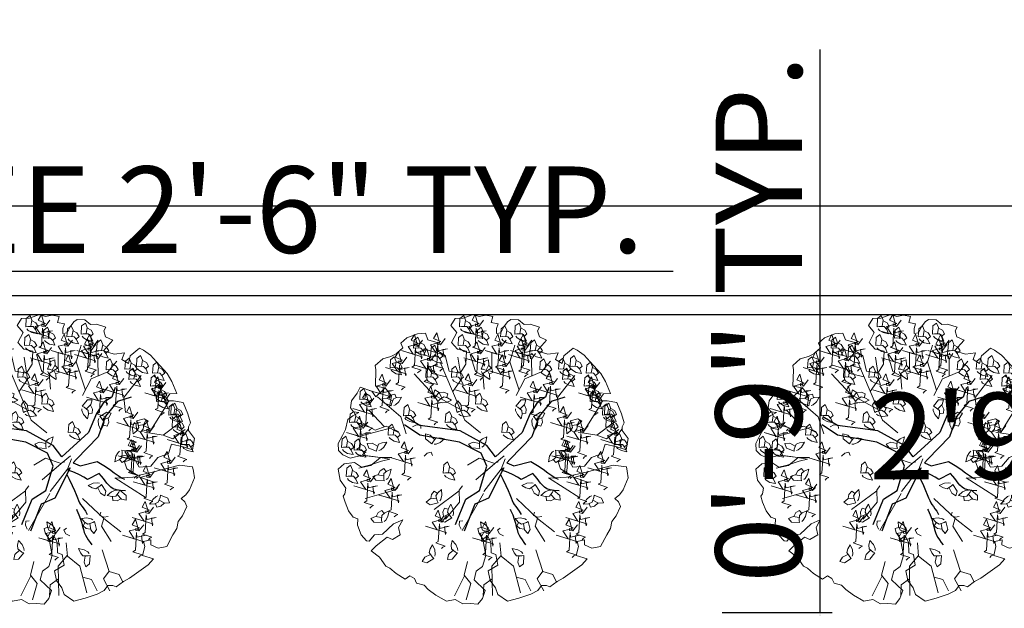
# Model space of a CAD drawing. Units: inches. Extents: x 2831 to 4250, y 1103 to 1797.
# Tile 5 of 15: x 3512 to 3614, y 1690 to 1751. Entities that reach past the tile are written whole.
import ezdxf

# ---------------------------------------------------------------- set-up
doc = ezdxf.new("R2010")
doc.units = ezdxf.units.IN
for name, color, linetype, lineweight in [('A-ANNO-DIMS', 2, 'Continuous', 18), ('A-ANNO-TEXT', 7, 'Continuous', 18), ('A-WALL-PATT', 252, 'Continuous', 13), ('ARBOL', 30, 'Continuous', 13), ('C-PROP', 7, 'Continuous', 25)]:
    doc.layers.add(name, color=color, linetype=linetype, lineweight=lineweight)
doc.layers.add('TALLO', color=36, linetype='Continuous')
doc.styles.get("Standard").update_dxf_attribs({"font": 'arial.ttf'})
doc.dimstyles.new('ISO-25', dxfattribs={"dimtxt": 9, "dimasz": 2.5, "dimexe": 1.25, "dimexo": 0.625, "dimtad": 1, "dimdec": 1, "dimlunit": 3, "dimtxsty": 'Standard', "dimcen": 2.5, "dimadec": 0, "dimazin": 0, "dimtfac": 1, "dimtdec": 1, "dimtmove": 0, "dimatfit": 3, "dimfxl": 1, "dimarcsym": 0})

# ---------------------------------------------------------------- blocks, each defined once
blk = doc.blocks.new('*D5')
at = {"layer": 'A-ANNO-DIMS', "color": 0, "lineweight": -2, "transparency": 16777216}
for p, q in [((3443.23, 1723.14), (3443.23, 1733.1)), ((3803.23, 1723.14), (3803.23, 1733.1)), ((3445.73, 1731.85), (3800.73, 1731.85))]:
    blk.add_line(p, q, dxfattribs=at)
at = {"layer": 'A-ANNO-DIMS', "color": 0, "transparency": 16777216}
for points in [[(3445.73, 1732.27), (3445.73, 1731.43), (3443.23, 1731.85)], [(3800.73, 1732.27), (3800.73, 1731.43), (3803.23, 1731.85)]]:
    blk.add_solid(points, dxfattribs=at)
at = {"layer": 'Defpoints', "color": 0, "transparency": 16777216}
for p in [(3803.23, 1731.85), (3443.23, 1722.51), (3803.23, 1722.51)]:
    blk.add_point(p, dxfattribs=at)
at = {"layer": 'A-ANNO-DIMS', "color": 0, "transparency": 16777216, "insert": (3623.23, 1737.07), "char_height": 9, "attachment_point": 5}
blk.add_mtext("30'", dxfattribs=at)
blk = doc.blocks.new('fresno')
at = {"layer": 'ARBOL'}
for p, q in [((2.96, 0.991), (3.575, 1.984)), ((-3.638, 1.194), (-4.164, 1.76)), ((-1.151, -0.932), (-1.99, -1.556)), ((-0.974, -3.757), (-1.31, -4.423))]:
    blk.add_line(p, q, dxfattribs=at)
blk.add_lwpolyline([(0.823, 4.745), (0.566, 4.764), (0.459, 4.687), (0.336, 4.518), (0.233, 4.322), (0.087, 4.298), (0.091, 4.464), (0.14, 4.621), (-0.09, 4.659), (-0.033, 4.863), (-0.264, 4.901), (-0.483, 4.866), (-0.686, 4.924), (-1.021, 4.801), (-1.288, 4.8), (-1.431, 4.563), (-1.234, 4.327), (-1.406, 4), (-1.205, 3.778), (-0.909, 3.705), (-0.931, 3.283), (-1.122, 2.983), (-1.491, 3.043), (-1.619, 3.562), (-1.9, 3.727), (-1.851, 3.982), (-2.197, 4.084), (-2.278, 4.31), (-2.543, 4.283), (-2.896, 4.152), (-3.091, 3.971), (-3.022, 3.817), (-3.244, 3.617), (-3.424, 3.528), (-3.697, 3.455), (-3.946, 3.236), (-3.922, 3.09), (-3.94, 2.548), (-3.617, 2.495), (-3.927, 2.19), (-4.062, 2.379), (-4.443, 2.512), (-4.546, 2.316), (-4.73, 2.062), (-4.767, 1.832), (-4.671, 1.698), (-4.486, 1.667), (-4.693, 1.559), (-4.854, 1.444), (-4.934, 1.102), (-5.037, 0.905), (-5.175, 0.644), (-5.166, 0.406), (-5.024, 0.264), (-4.781, 0.153), (-4.363, 0.249), (-4.014, 0.215), (-3.783, 0.177), (-3.46, 0.124), (-3.733, 0.051), (-4.132, -0.073), (-4.404, -0.146), (-4.639, 0.011), (-4.977, -0.028), (-5.172, -0.209), (-5.113, -0.574), (-4.921, -0.843), (-4.951, -1.027), (-5.012, -1.112), (-4.95, -1.311), (-4.83, -1.592), (-4.676, -1.807), (-4.518, -1.856), (-4.529, -2.068), (-4.417, -2.394), (-4.236, -2.59), (-4.143, -2.605), (-3.967, -2.397), (-3.703, -2.37), (-3.339, -2.027), (-3.032, -1.889), (-3.169, -2.15), (-3.115, -2.396), (-3.376, -2.542), (-3.552, -2.466), (-3.909, -2.762), (-4.077, -2.924), (-3.804, -3.135), (-3.592, -3.43), (-3.461, -3.499), (-3.253, -3.676), (-2.953, -3.867), (-2.792, -3.752), (-2.642, -3.848), (-2.572, -4.001), (-2.323, -4.066), (-2.18, -4.208), (-1.926, -4.392), (-1.58, -4.591), (-1.288, -4.545), (-1.027, -4.683), (-0.788, -4.675), (-0.531, -4.693), (-0.382, -4.505), (-0.29, -4.236), (-0.66, -3.891), (-0.588, -3.595), (-0.374, -3.441), (-0.267, -3.079), (-0.368, -2.541), (-0.208, -2.426), (-0.099, -2.633), (-0.087, -2.991), (0.071, -3.04), (0.129, -3.405), (-0.185, -3.59), (-0.119, -3.909), (0.055, -4.151), (0.136, -4.377), (0.456, -4.596), (0.828, -4.491), (1.227, -4.368), (1.461, -4.241), (1.583, -4.071), (1.748, -4.075), (1.86, -4.117), (2.101, -3.944), (2.308, -3.836), (2.925, -3.393), (3.101, -3.185), (2.74, -3.078), (2.812, -2.782), (2.769, -2.61), (3.015, -2.555), (3.012, -2.721), (3.254, -2.832), (3.546, -2.785), (3.752, -2.393), (3.882, -2.177), (3.92, -1.947), (4.069, -1.758), (4.214, -1.451), (4.144, -1.297), (4.021, -1.182), (4.182, -1.067), (4.304, -0.897), (4.464, -0.497), (4.429, -0.279), (4.406, -0.133), (3.964, -0.083), (3.074, -0.315), (2.582, -0.424), (2.217, -0.197), (2.136, 0.029), (2.462, 0.141), (2.628, -0.147), (3.012, -0.116), (3.249, 0.177), (3.602, 0.308), (3.701, 0.623), (4.089, 0.535), (4.404, 0.436), (4.464, 0.805), (4.272, 1.074), (4.267, 1.193), (4.336, 1.324), (4.243, 1.623), (4.092, 2.003), (3.769, 2.057), (3.485, 2.056), (3.642, 2.291), (3.88, 2.299), (3.71, 2.706), (3.563, 2.967), (3.201, 3.358), (3.001, 3.581), (2.766, 3.738), (2.635, 3.807), (2.332, 3.549), (2.268, 3.299), (2.052, 3.429), (2.136, 3.652), (1.798, 3.613), (1.437, 3.72), (1.755, 4.071), (1.513, 4.182), (1.451, 4.381), (1.519, 4.512), (1.204, 4.611), (1.012, 4.596)], close=True, dxfattribs=at)
for points in [[(-0.346, 4.735), (-0.501, 4.528), (-0.605, 4.545), (-0.605, 4.614), (-0.519, 4.563), (-0.622, 4.925), (-0.726, 4.735), (-0.484, 4.632), (-0.622, 4.58), (-0.829, 4.528), (-0.657, 4.27), (-1.053, 4.39), (-0.363, 4.183), (-0.381, 4.114), (-0.415, 4.373), (-0.26, 4.39), (-0.57, 4.321), (-0.588, 4.476), (-0.622, 3.89), (-0.708, 3.839), (-0.398, 3.735), (-0.467, 3.701), (-0.519, 3.649)], [(-1.104, 4.45), (-1.063, 4.399), (-0.939, 4.325), (-0.757, 4.285), (-0.82, 4.431), (-0.903, 4.527), (-1.075, 4.533), (-1.143, 4.521), (-1.126, 4.792), (-1.002, 4.891), (-0.939, 4.738), (-0.975, 4.535)], [(-0.935, 4.717), (-0.809, 4.65), (-0.736, 4.529), (-0.824, 4.459)], [(0.734, 4.203), (0.775, 4.152), (0.9, 4.078), (1.082, 4.038), (1.018, 4.185), (0.936, 4.281), (0.763, 4.287), (0.696, 4.274), (0.712, 4.546), (0.837, 4.645), (0.899, 4.491), (0.863, 4.289)], [(-2.368, 4.073), (-2.523, 3.866), (-2.627, 3.883), (-2.627, 3.952), (-2.541, 3.9), (-2.644, 4.262), (-2.748, 4.073), (-2.506, 3.969), (-2.644, 3.918), (-2.851, 3.866), (-2.679, 3.607), (-3.075, 3.728), (-2.385, 3.521), (-2.403, 3.452), (-2.437, 3.711), (-2.282, 3.728), (-2.592, 3.659), (-2.61, 3.814), (-2.644, 3.228), (-2.73, 3.176), (-2.42, 3.073), (-2.489, 3.038), (-2.541, 2.987)], [(-1.623, 4.132), (-1.778, 3.925), (-1.882, 3.942), (-1.882, 4.011), (-1.795, 3.959), (-1.899, 4.321), (-2.002, 4.132), (-1.761, 4.028), (-1.899, 3.977), (-2.106, 3.925), (-1.933, 3.666), (-2.33, 3.787), (-1.64, 3.58), (-1.657, 3.511), (-1.692, 3.77), (-1.537, 3.787), (-1.847, 3.718), (-1.864, 3.873), (-1.899, 3.287), (-1.985, 3.235), (-1.675, 3.132), (-1.744, 3.097), (-1.795, 3.046)], [(-1.149, 3.822), (-1.108, 3.771), (-0.983, 3.697), (-0.802, 3.657), (-0.865, 3.804), (-0.948, 3.9), (-1.12, 3.906), (-1.188, 3.893), (-1.171, 4.165), (-1.047, 4.264), (-0.984, 4.111), (-1.02, 3.908)], [(-0.521, 4.069), (-0.48, 4.018), (-0.356, 3.944), (-0.174, 3.904), (-0.237, 4.051), (-0.32, 4.146), (-0.492, 4.152), (-0.56, 4.14), (-0.543, 4.411), (-0.419, 4.511), (-0.356, 4.357), (-0.392, 4.154)], [(-0.352, 4.337), (-0.226, 4.269), (-0.153, 4.148), (-0.241, 4.078)], [(0.413, 4.08), (0.258, 3.873), (0.154, 3.89), (0.154, 3.959), (0.241, 3.908), (0.137, 4.27), (0.034, 4.08), (0.275, 3.977), (0.137, 3.925), (-0.07, 3.873), (0.103, 3.614), (-0.294, 3.735), (0.396, 3.528), (0.379, 3.459), (0.344, 3.718), (0.499, 3.735), (0.189, 3.666), (0.172, 3.821), (0.137, 3.235), (0.051, 3.183), (0.361, 3.08), (0.292, 3.046), (0.241, 2.994)], [(0.263, 4.114), (0.304, 4.063), (0.429, 3.989), (0.611, 3.948), (0.547, 4.095), (0.465, 4.191), (0.293, 4.197), (0.225, 4.185), (0.242, 4.456), (0.366, 4.555), (0.428, 4.402), (0.393, 4.199)], [(0.433, 4.381), (0.558, 4.314), (0.631, 4.193), (0.544, 4.122)], [(1.259, 4.08), (1.103, 3.873), (1, 3.89), (1, 3.959), (1.086, 3.908), (0.982, 4.27), (0.879, 4.08), (1.12, 3.977), (0.982, 3.925), (0.775, 3.873), (0.948, 3.614), (0.551, 3.735), (1.241, 3.528), (1.224, 3.459), (1.189, 3.718), (1.345, 3.735), (1.034, 3.666), (1.017, 3.821), (0.982, 3.235), (0.896, 3.183), (1.207, 3.08), (1.138, 3.046), (1.086, 2.994)], [(0.904, 4.471), (1.029, 4.404), (1.102, 4.282), (1.015, 4.212)], [(-2.629, 3.733), (-2.588, 3.682), (-2.463, 3.608), (-2.281, 3.568), (-2.345, 3.715), (-2.427, 3.81), (-2.6, 3.816), (-2.667, 3.804), (-2.651, 4.075), (-2.526, 4.175), (-2.464, 4.021), (-2.5, 3.818)], [(-2.459, 4), (-2.334, 3.933), (-2.261, 3.812), (-2.348, 3.742)], [(-0.287, 3.833), (-0.442, 3.626), (-0.546, 3.643), (-0.546, 3.712), (-0.46, 3.661), (-0.563, 4.023), (-0.667, 3.833), (-0.425, 3.73), (-0.563, 3.678), (-0.77, 3.626), (-0.598, 3.367), (-0.995, 3.488), (-0.304, 3.281), (-0.322, 3.212), (-0.356, 3.471), (-0.201, 3.488), (-0.511, 3.419), (-0.529, 3.574), (-0.563, 2.988), (-0.649, 2.936), (-0.339, 2.833), (-0.408, 2.799), (-0.46, 2.747)], [(-0.98, 4.09), (-0.854, 4.023), (-0.781, 3.901), (-0.869, 3.831)], [(1.189, 3.942), (1.034, 3.735), (0.931, 3.752), (0.931, 3.821), (1.017, 3.77), (0.913, 4.132), (0.81, 3.942), (1.051, 3.839), (0.913, 3.787), (0.706, 3.735), (0.879, 3.477), (0.482, 3.597), (1.172, 3.39), (1.155, 3.321), (1.12, 3.58), (1.276, 3.597), (0.965, 3.528), (0.948, 3.683), (0.913, 3.097), (0.827, 3.046), (1.138, 2.942), (1.069, 2.908), (1.017, 2.856)], [(1.25, 3.643), (1.291, 3.592), (1.416, 3.518), (1.597, 3.478), (1.534, 3.625), (1.451, 3.721), (1.279, 3.727), (1.211, 3.714), (1.228, 3.985), (1.352, 4.085), (1.415, 3.931), (1.379, 3.729)], [(-2.898, 3.511), (-3.053, 3.304), (-3.157, 3.321), (-3.157, 3.39), (-3.071, 3.339), (-3.174, 3.701), (-3.278, 3.511), (-3.036, 3.408), (-3.174, 3.356), (-3.381, 3.304), (-3.209, 3.046), (-3.605, 3.166), (-2.915, 2.959), (-2.932, 2.89), (-2.967, 3.149), (-2.812, 3.166), (-3.122, 3.097), (-3.14, 3.253), (-3.174, 2.666), (-3.26, 2.615), (-2.95, 2.511), (-3.019, 2.477), (-3.071, 2.425)], [(-1.951, 3.597), (-2.106, 3.39), (-2.209, 3.408), (-2.209, 3.477), (-2.123, 3.425), (-2.227, 3.787), (-2.33, 3.597), (-2.089, 3.494), (-2.227, 3.442), (-2.434, 3.39), (-2.261, 3.132), (-2.658, 3.252), (-1.968, 3.046), (-1.985, 2.977), (-2.02, 3.235), (-1.864, 3.252), (-2.175, 3.183), (-2.192, 3.339), (-2.227, 2.752), (-2.313, 2.701), (-2.002, 2.597), (-2.071, 2.563), (-2.123, 2.511)], [(-2.068, 3.464), (-2.027, 3.413), (-1.903, 3.339), (-1.721, 3.299), (-1.784, 3.446), (-1.867, 3.542), (-2.039, 3.547), (-2.107, 3.535), (-2.09, 3.806), (-1.966, 3.906), (-1.903, 3.752), (-1.939, 3.55)], [(-1.899, 3.732), (-1.773, 3.664), (-1.7, 3.543), (-1.788, 3.473)], [(-0.063, 3.671), (-0.069, 3.151), (-0.364, 2.965), (-0.319, 2.449)], [(0.837, 2.414), (0.533, 3.352), (0.697, 3.906)], [(1.259, 2.882), (1.254, 3.446), (1.381, 3.636)], [(1.419, 3.911), (1.545, 3.844), (1.618, 3.722), (1.53, 3.652)], [(-3.413, 3.083), (-3.373, 3.032), (-3.248, 2.958), (-3.066, 2.918), (-3.129, 3.065), (-3.212, 3.161), (-3.384, 3.167), (-3.452, 3.154), (-3.435, 3.425), (-3.311, 3.525), (-3.248, 3.371), (-3.284, 3.169)], [(-3.244, 3.351), (-3.118, 3.284), (-3.045, 3.162), (-3.133, 3.092)], [(-0.448, 1), (-0.961, 1.419), (-1.784, 3.341)], [(-1.367, 2.367), (-1.081, 2.78), (-1.193, 3.514)], [(-0.923, 3.449), (-0.951, 3.425), (-0.93, 3.313)], [(-0.358, 2.895), (-0.615, 3.037), (-0.783, 3.596)], [(-0.41, 3.035), (-0.387, 2.974), (-0.291, 2.865), (-0.131, 2.771), (-0.146, 2.93), (-0.195, 3.047), (-0.357, 3.106), (-0.425, 3.115), (-0.325, 3.368), (-0.176, 3.424), (-0.164, 3.258), (-0.261, 3.077)], [(0.558, 3.402), (0.403, 3.195), (0.299, 3.212), (0.299, 3.281), (0.386, 3.23), (0.282, 3.592), (0.179, 3.402), (0.42, 3.299), (0.282, 3.247), (0.075, 3.195), (0.248, 2.936), (-0.149, 3.057), (0.541, 2.85), (0.524, 2.781), (0.489, 3.04), (0.644, 3.057), (0.334, 2.988), (0.317, 3.143), (0.282, 2.557), (0.196, 2.505), (0.506, 2.402), (0.437, 2.368), (0.386, 2.316)], [(0.746, 2.242), (1.034, 2.786), (1.584, 3.019), (1.879, 3.374)], [(1.564, 3.016), (1.605, 2.965), (1.729, 2.891), (1.911, 2.851), (1.848, 2.998), (1.765, 3.094), (1.593, 3.099), (1.525, 3.087), (1.542, 3.358), (1.666, 3.458), (1.729, 3.304), (1.693, 3.102)], [(1.733, 3.284), (1.859, 3.216), (1.932, 3.095), (1.844, 3.025)], [(2.191, 3.038), (2.232, 2.987), (2.357, 2.913), (2.539, 2.873), (2.475, 3.02), (2.393, 3.116), (2.221, 3.122), (2.153, 3.109), (2.17, 3.381), (2.294, 3.48), (2.356, 3.326), (2.321, 3.124)], [(2.361, 3.306), (2.486, 3.239), (2.559, 3.117), (2.472, 3.047)], [(2.573, 3.128), (2.613, 3.077), (2.738, 3.003), (2.92, 2.963), (2.857, 3.11), (2.774, 3.205), (2.602, 3.211), (2.534, 3.199), (2.551, 3.47), (2.675, 3.57), (2.738, 3.416), (2.702, 3.214)], [(2.742, 3.396), (2.868, 3.328), (2.941, 3.207), (2.853, 3.137)], [(3.111, 2.904), (3.152, 2.853), (3.276, 2.779), (3.458, 2.739), (3.395, 2.886), (3.312, 2.981), (3.14, 2.987), (3.072, 2.975), (3.089, 3.246), (3.213, 3.346), (3.276, 3.192), (3.24, 2.99)], [(-1.112, 1.773), (-2.014, 2.265), (-2.654, 2.957)], [(-2.225, 2.77), (-2.184, 2.718), (-2.06, 2.645), (-1.878, 2.604), (-1.941, 2.751), (-2.024, 2.847), (-2.196, 2.853), (-2.264, 2.84), (-2.247, 3.112), (-2.123, 3.211), (-2.06, 3.058), (-2.096, 2.855)], [(-1.575, 2.854), (-2.052, 2.969), (-2.2, 3.178)], [(-2.056, 3.037), (-1.93, 2.97), (-1.857, 2.849), (-1.945, 2.778)], [(-1.373, 2.77), (-1.332, 2.718), (-1.208, 2.645), (-1.026, 2.604), (-1.089, 2.751), (-1.172, 2.847), (-1.344, 2.853), (-1.412, 2.84), (-1.395, 3.112), (-1.271, 3.211), (-1.208, 3.058), (-1.244, 2.855)], [(-0.57, 2.77), (-0.726, 2.563), (-0.829, 2.58), (-0.829, 2.649), (-0.743, 2.597), (-0.846, 2.959), (-0.95, 2.77), (-0.708, 2.666), (-0.846, 2.615), (-1.053, 2.563), (-0.881, 2.304), (-1.278, 2.425), (-0.588, 2.218), (-0.605, 2.149), (-0.639, 2.408), (-0.484, 2.425), (-0.795, 2.356), (-0.812, 2.511), (-0.846, 1.925), (-0.933, 1.873), (-0.622, 1.77), (-0.691, 1.735), (-0.743, 1.684)], [(-1.204, 3.037), (-1.078, 2.97), (-1.005, 2.849), (-1.093, 2.778)], [(-0.166, 3.238), (-0.068, 3.135), (-0.036, 2.997), (-0.141, 2.957)], [(2.121, 2.804), (1.966, 2.597), (1.862, 2.615), (1.862, 2.683), (1.949, 2.632), (1.845, 2.994), (1.742, 2.804), (1.983, 2.701), (1.845, 2.649), (1.638, 2.597), (1.811, 2.339), (1.414, 2.459), (2.104, 2.252), (2.087, 2.184), (2.052, 2.442), (2.207, 2.459), (1.897, 2.39), (1.88, 2.546), (1.845, 1.959), (1.759, 1.908), (2.069, 1.804), (2, 1.77), (1.949, 1.718)], [(2.326, 2.702), (2.367, 2.651), (2.492, 2.577), (2.673, 2.537), (2.61, 2.684), (2.527, 2.78), (2.355, 2.786), (2.287, 2.773), (2.304, 3.045), (2.428, 3.144), (2.491, 2.99), (2.455, 2.788)], [(2.495, 2.97), (2.621, 2.903), (2.694, 2.781), (2.606, 2.711)], [(3.28, 3.172), (3.406, 3.104), (3.479, 2.983), (3.391, 2.913)], [(-3.434, 2.752), (-3.59, 2.546), (-3.693, 2.563), (-3.693, 2.632), (-3.607, 2.58), (-3.71, 2.942), (-3.814, 2.752), (-3.572, 2.649), (-3.71, 2.597), (-3.917, 2.546), (-3.745, 2.287), (-4.142, 2.408), (-3.452, 2.201), (-3.469, 2.132), (-3.503, 2.39), (-3.348, 2.408), (-3.659, 2.339), (-3.676, 2.494), (-3.71, 1.908), (-3.797, 1.856), (-3.486, 1.753), (-3.555, 1.718), (-3.607, 1.666)], [(1.586, 2.528), (1.431, 2.321), (1.327, 2.339), (1.327, 2.408), (1.414, 2.356), (1.31, 2.718), (1.207, 2.528), (1.448, 2.425), (1.31, 2.373), (1.103, 2.321), (1.276, 2.063), (0.879, 2.184), (1.569, 1.977), (1.552, 1.908), (1.517, 2.166), (1.673, 2.184), (1.362, 2.115), (1.345, 2.27), (1.31, 1.684), (1.224, 1.632), (1.535, 1.528), (1.466, 1.494), (1.414, 1.442)], [(2.171, 1.674), (2.121, 2.172), (2.689, 2.898)], [(3.519, 2.666), (3.363, 2.459), (3.26, 2.477), (3.26, 2.546), (3.346, 2.494), (3.243, 2.856), (3.139, 2.666), (3.381, 2.563), (3.243, 2.511), (3.036, 2.459), (3.208, 2.201), (2.811, 2.321), (3.501, 2.115), (3.484, 2.046), (3.45, 2.304), (3.605, 2.321), (3.294, 2.252), (3.277, 2.408), (3.243, 1.821), (3.156, 1.77), (3.467, 1.666), (3.398, 1.632), (3.346, 1.58)], [(3.043, 2.478), (3.084, 2.427), (3.209, 2.353), (3.391, 2.313), (3.327, 2.46), (3.245, 2.556), (3.073, 2.562), (3.005, 2.549), (3.022, 2.82), (3.146, 2.92), (3.208, 2.766), (3.173, 2.564)], [(3.213, 2.746), (3.338, 2.679), (3.411, 2.557), (3.324, 2.487)], [(-3.986, 2.149), (-4.142, 1.942), (-4.245, 1.959), (-4.245, 2.028), (-4.159, 1.977), (-4.262, 2.339), (-4.366, 2.149), (-4.124, 2.046), (-4.262, 1.994), (-4.47, 1.942), (-4.297, 1.684), (-4.694, 1.804), (-4.004, 1.597), (-4.021, 1.528), (-4.055, 1.787), (-3.9, 1.804), (-4.211, 1.735), (-4.228, 1.89), (-4.262, 1.304), (-4.349, 1.253), (-4.038, 1.149), (-4.107, 1.115), (-4.159, 1.063)], [(-4.422, 2.03), (-4.381, 1.979), (-4.257, 1.905), (-4.075, 1.865), (-4.138, 2.012), (-4.221, 2.108), (-4.393, 2.114), (-4.461, 2.101), (-4.444, 2.372), (-4.32, 2.472), (-4.257, 2.318), (-4.293, 2.116)], [(-4.253, 2.298), (-4.127, 2.231), (-4.054, 2.109), (-4.142, 2.039)], [(-3.468, 1.85), (-3.409, 2.222), (-3.628, 2.505)], [(-1.817, 2.351), (-1.972, 2.144), (-2.075, 2.162), (-2.075, 2.231), (-1.989, 2.179), (-2.093, 2.541), (-2.196, 2.351), (-1.955, 2.248), (-2.093, 2.196), (-2.3, 2.144), (-2.127, 1.886), (-2.524, 2.006), (-1.834, 1.8), (-1.851, 1.731), (-1.886, 1.989), (-1.73, 2.006), (-2.041, 1.937), (-2.058, 2.093), (-2.093, 1.506), (-2.179, 1.455), (-1.868, 1.351), (-1.937, 1.317), (-1.989, 1.265)], [(-1.786, 2.007), (-1.722, 1.99), (-1.578, 2.003), (-1.407, 2.078), (-1.545, 2.159), (-1.668, 2.188), (-1.811, 2.092), (-1.859, 2.042), (-2.004, 2.271), (-1.962, 2.425), (-1.821, 2.337), (-1.731, 2.152)], [(-1.806, 2.323), (-1.665, 2.343), (-1.534, 2.287), (-1.564, 2.179)], [(-0.566, 1.873), (-0.525, 1.822), (-0.4, 1.748), (-0.219, 1.708), (-0.282, 1.855), (-0.365, 1.951), (-0.537, 1.957), (-0.605, 1.944), (-0.588, 2.216), (-0.464, 2.315), (-0.401, 2.162), (-0.437, 1.959)], [(3.178, 2.165), (3.219, 2.113), (3.344, 2.04), (3.525, 1.999), (3.462, 2.146), (3.379, 2.242), (3.207, 2.248), (3.139, 2.236), (3.156, 2.507), (3.28, 2.606), (3.343, 2.453), (3.307, 2.25)], [(3.245, 1.963), (3.286, 1.912), (3.411, 1.838), (3.593, 1.798), (3.529, 1.945), (3.447, 2.041), (3.274, 2.046), (3.206, 2.034), (3.223, 2.305), (3.347, 2.405), (3.41, 2.251), (3.374, 2.049)], [(3.347, 2.432), (3.473, 2.365), (3.546, 2.244), (3.458, 2.173)], [(-2.916, 0.958), (-3.096, 1.528), (-3.871, 2.197)], [(-3.331, 1.905), (-3.269, 1.928), (-3.161, 2.024), (-3.066, 2.184), (-3.226, 2.169), (-3.342, 2.121), (-3.401, 1.958), (-3.41, 1.89), (-3.663, 1.99), (-3.719, 2.139), (-3.554, 2.151), (-3.372, 2.054)], [(-3.533, 2.149), (-3.43, 2.247), (-3.292, 2.279), (-3.252, 2.174)], [(-1.164, 1.612), (-1.109, 1.576), (-0.967, 1.544), (-0.782, 1.562), (-0.888, 1.682), (-0.996, 1.748), (-1.162, 1.7), (-1.222, 1.667), (-1.29, 1.93), (-1.203, 2.063), (-1.096, 1.937), (-1.067, 1.733)], [(-0.397, 2.141), (-0.271, 2.074), (-0.198, 1.952), (-0.286, 1.882)], [(0.72, 1.798), (0.723, 1.733), (0.781, 1.6), (0.904, 1.46), (0.939, 1.616), (0.929, 1.742), (0.793, 1.848), (0.73, 1.878), (0.904, 2.088), (1.062, 2.095), (1.023, 1.934), (0.875, 1.791)], [(3.415, 2.231), (3.54, 2.163), (3.613, 2.042), (3.525, 1.972)], [(3.716, 1.537), (3.757, 1.486), (3.882, 1.412), (4.063, 1.372), (4, 1.519), (3.917, 1.615), (3.745, 1.621), (3.677, 1.608), (3.694, 1.88), (3.818, 1.979), (3.881, 1.825), (3.845, 1.623)], [(-4.759, 1.269), (-4.718, 1.217), (-4.593, 1.144), (-4.411, 1.103), (-4.475, 1.25), (-4.557, 1.346), (-4.729, 1.352), (-4.797, 1.339), (-4.78, 1.611), (-4.656, 1.71), (-4.594, 1.557), (-4.629, 1.354)], [(-2.965, 1.493), (-2.924, 1.441), (-2.799, 1.368), (-2.618, 1.327), (-2.681, 1.474), (-2.764, 1.57), (-2.936, 1.576), (-3.004, 1.564), (-2.987, 1.835), (-2.863, 1.934), (-2.8, 1.781), (-2.836, 1.578)], [(-2.796, 1.76), (-2.67, 1.693), (-2.597, 1.572), (-2.685, 1.501)], [(-1.575, 1.269), (-1.534, 1.217), (-1.409, 1.144), (-1.228, 1.103), (-1.291, 1.25), (-1.373, 1.346), (-1.546, 1.352), (-1.614, 1.339), (-1.597, 1.611), (-1.473, 1.71), (-1.41, 1.557), (-1.446, 1.354)], [(-1.085, 1.919), (-0.945, 1.893), (-0.838, 1.801), (-0.9, 1.707)], [(1.014, 1.915), (1.077, 1.787), (1.064, 1.646), (0.952, 1.64)], [(1.283, 1.469), (1.266, 1.405), (1.279, 1.261), (1.354, 1.09), (1.435, 1.228), (1.464, 1.351), (1.368, 1.494), (1.318, 1.542), (1.547, 1.687), (1.7, 1.645), (1.613, 1.504), (1.428, 1.414)], [(2.587, 1.684), (2.432, 1.477), (2.328, 1.494), (2.328, 1.563), (2.414, 1.511), (2.311, 1.873), (2.207, 1.684), (2.449, 1.58), (2.311, 1.528), (2.104, 1.477), (2.276, 1.218), (1.88, 1.339), (2.57, 1.132), (2.552, 1.063), (2.518, 1.321), (2.673, 1.339), (2.363, 1.27), (2.345, 1.425), (2.311, 0.839), (2.225, 0.787), (2.535, 0.684), (2.466, 0.649), (2.414, 0.597)], [(3.649, 1.515), (3.69, 1.464), (3.814, 1.39), (3.996, 1.35), (3.933, 1.497), (3.85, 1.592), (3.678, 1.598), (3.61, 1.586), (3.627, 1.857), (3.751, 1.957), (3.814, 1.803), (3.778, 1.601)], [(3.818, 1.783), (3.944, 1.715), (4.017, 1.594), (3.929, 1.524)], [(3.885, 1.805), (4.011, 1.738), (4.084, 1.616), (3.996, 1.546)], [(-4.193, 1.356), (-4.349, 1.149), (-4.452, 1.166), (-4.452, 1.235), (-4.366, 1.184), (-4.469, 1.546), (-4.573, 1.356), (-4.331, 1.253), (-4.469, 1.201), (-4.677, 1.149), (-4.504, 0.89), (-4.901, 1.011), (-4.211, 0.804), (-4.228, 0.735), (-4.262, 0.994), (-4.107, 1.011), (-4.418, 0.942), (-4.435, 1.097), (-4.469, 0.511), (-4.556, 0.459), (-4.245, 0.356), (-4.314, 0.322), (-4.366, 0.27)], [(-4.589, 1.536), (-4.464, 1.469), (-4.391, 1.348), (-4.478, 1.277)], [(-3.192, 1.017), (-3.578, 1.215), (-3.949, 1.081), (-4.398, 1.339)], [(-1.406, 1.536), (-1.28, 1.469), (-1.207, 1.348), (-1.295, 1.277)], [(0.308, 0.933), (0.349, 0.881), (0.474, 0.807), (0.656, 0.767), (0.592, 0.914), (0.51, 1.01), (0.337, 1.016), (0.27, 1.003), (0.286, 1.275), (0.411, 1.374), (0.473, 1.221), (0.437, 1.018)], [(1.599, 1.489), (1.618, 1.348), (1.563, 1.217), (1.455, 1.247)], [(2.479, 1.34), (2.443, 1.285), (2.411, 1.143), (2.429, 0.958), (2.549, 1.064), (2.615, 1.172), (2.567, 1.338), (2.534, 1.398), (2.797, 1.466), (2.93, 1.379), (2.804, 1.272), (2.6, 1.243)], [(3.139, 1.235), (2.984, 1.028), (2.88, 1.046), (2.88, 1.115), (2.967, 1.063), (2.863, 1.425), (2.759, 1.235), (3.001, 1.132), (2.863, 1.08), (2.656, 1.028), (2.828, 0.77), (2.432, 0.891), (3.122, 0.684), (3.105, 0.615), (3.07, 0.873), (3.225, 0.891), (2.915, 0.822), (2.897, 0.977), (2.863, 0.391), (2.777, 0.339), (3.087, 0.235), (3.018, 0.201), (2.967, 0.149)], [(4.01, 1.36), (3.422, 0.918)], [(3.761, 1.112), (3.802, 1.061), (3.926, 0.987), (4.108, 0.947), (4.045, 1.093), (3.962, 1.189), (3.79, 1.195), (3.722, 1.183), (3.739, 1.454), (3.863, 1.553), (3.926, 1.4), (3.89, 1.197)], [(3.93, 1.379), (4.056, 1.312), (4.129, 1.191), (4.041, 1.121)], [(-3.354, 1.176), (-4.529, 0.864)], [(-3.481, 0.843), (-3.44, 0.792), (-3.315, 0.718), (-3.133, 0.678), (-3.197, 0.825), (-3.279, 0.92), (-3.451, 0.926), (-3.519, 0.914), (-3.502, 1.185), (-3.378, 1.285), (-3.316, 1.131), (-3.351, 0.928)], [(-3.311, 1.111), (-3.186, 1.043), (-3.113, 0.922), (-3.2, 0.852)], [(-2.703, 1.201), (-2.575, 1.263), (-2.433, 1.251), (-2.428, 1.139)], [(0.478, 1.2), (0.603, 1.133), (0.676, 1.011), (0.589, 0.941)], [(2.786, 1.261), (2.76, 1.121), (2.668, 1.014), (2.574, 1.076)], [(2.808, 1.015), (3.422, 0.918), (3.422, 0.918), (3.748, 0.794), (4.154, 1.111)], [(4.26, 1.115), (4.105, 0.908), (4.002, 0.925), (4.002, 0.994), (4.088, 0.942), (3.984, 1.304), (3.881, 1.115), (4.122, 1.011), (3.984, 0.959), (3.777, 0.908), (3.95, 0.649), (3.553, 0.77), (4.243, 0.563), (4.226, 0.494), (4.191, 0.753), (4.347, 0.77), (4.036, 0.701), (4.019, 0.856), (3.984, 0.27), (3.898, 0.218), (4.209, 0.115), (4.14, 0.08), (4.088, 0.029)], [(-5.028, 0.44), (-4.987, 0.388), (-4.862, 0.315), (-4.68, 0.274), (-4.744, 0.421), (-4.826, 0.517), (-4.998, 0.523), (-5.066, 0.511), (-5.049, 0.782), (-4.925, 0.881), (-4.863, 0.728), (-4.898, 0.525)], [(-4.858, 0.707), (-4.733, 0.64), (-4.66, 0.519), (-4.747, 0.448)], [(-4.602, 0.35), (-4.561, 0.299), (-4.436, 0.225), (-4.254, 0.185), (-4.318, 0.332), (-4.4, 0.428), (-4.572, 0.433), (-4.64, 0.421), (-4.623, 0.692), (-4.499, 0.792), (-4.437, 0.638), (-4.472, 0.436)], [(-3.824, 0.404), (-3.763, 0.427), (-3.654, 0.523), (-3.559, 0.683), (-3.719, 0.668), (-3.835, 0.62), (-3.894, 0.457), (-3.903, 0.389), (-4.156, 0.489), (-4.212, 0.638), (-4.047, 0.65), (-3.865, 0.553)], [(-2.698, 0.509), (-2.854, 0.302), (-2.957, 0.319), (-2.957, 0.388), (-2.871, 0.336), (-2.974, 0.698), (-3.078, 0.509), (-2.836, 0.405), (-2.974, 0.353), (-3.182, 0.302), (-3.009, 0.043), (-3.406, 0.164), (-2.716, -0.043), (-2.733, -0.112), (-2.767, 0.147), (-2.612, 0.164), (-2.923, 0.095), (-2.94, 0.25), (-2.974, -0.336), (-3.061, -0.388), (-2.75, -0.491), (-2.819, -0.526), (-2.871, -0.577)], [(-1.981, 0.615), (-1.915, 0.618), (-1.782, 0.676), (-1.643, 0.799), (-1.799, 0.834), (-1.925, 0.824), (-2.031, 0.688), (-2.061, 0.626), (-2.27, 0.799), (-2.278, 0.958), (-2.117, 0.918), (-1.974, 0.77)], [(-0.397, 0.517), (-0.346, 0.557), (-0.272, 0.682), (-0.232, 0.864), (-0.379, 0.801), (-0.474, 0.718), (-0.48, 0.546), (-0.468, 0.478), (-0.739, 0.495), (-0.838, 0.619), (-0.685, 0.682), (-0.482, 0.646)], [(2.639, 0.58), (2.483, 0.373), (2.38, 0.391), (2.38, 0.46), (2.466, 0.408), (2.363, 0.77), (2.259, 0.58), (2.501, 0.477), (2.363, 0.425), (2.156, 0.373), (2.328, 0.115), (1.931, 0.235), (2.621, 0.029), (2.604, -0.04), (2.57, 0.218), (2.725, 0.235), (2.414, 0.166), (2.397, 0.322), (2.363, -0.265), (2.276, -0.316), (2.587, -0.42), (2.518, -0.454), (2.466, -0.506)], [(2.708, 0.563), (2.552, 0.356), (2.449, 0.373), (2.449, 0.442), (2.535, 0.391), (2.432, 0.753), (2.328, 0.563), (2.57, 0.46), (2.432, 0.408), (2.225, 0.356), (2.397, 0.097), (2, 0.218), (2.69, 0.011), (2.673, -0.058), (2.639, 0.201), (2.794, 0.218), (2.483, 0.149), (2.466, 0.304), (2.432, -0.282), (2.345, -0.334), (2.656, -0.437), (2.587, -0.471), (2.535, -0.523)], [(4.075, 0.529), (4.116, 0.478), (4.24, 0.404), (4.422, 0.364), (4.359, 0.511), (4.276, 0.607), (4.104, 0.613), (4.036, 0.6), (4.053, 0.871), (4.177, 0.971), (4.24, 0.817), (4.204, 0.615)], [(4.244, 0.797), (4.37, 0.73), (4.443, 0.608), (4.355, 0.538)], [(-4.432, 0.618), (-4.307, 0.55), (-4.234, 0.429), (-4.321, 0.359)], [(-2.322, 0.222), (-2.219, 0.321), (-2.081, 0.353), (-2.042, 0.248)], [(1.978, 0.384), (1.927, 0.343), (1.853, 0.218), (1.813, 0.036), (1.96, 0.1), (2.056, 0.182), (2.061, 0.355), (2.049, 0.422), (2.32, 0.406), (2.42, 0.281), (2.266, 0.219), (2.064, 0.254)], [(3.829, 0.184), (3.674, -0.023), (3.57, -0.006), (3.57, 0.063), (3.657, 0.011), (3.553, 0.373), (3.45, 0.184), (3.691, 0.08), (3.553, 0.029), (3.346, -0.023), (3.519, -0.282), (3.122, -0.161), (3.812, -0.368), (3.795, -0.437), (3.76, -0.178), (3.915, -0.161), (3.605, -0.23), (3.588, -0.075), (3.553, -0.661), (3.467, -0.713), (3.777, -0.816), (3.708, -0.851), (3.657, -0.902)], [(-3.394, 0.18), (-3.77, 0.182), (-4.532, 0.27)], [(-3.77, 0.182), (-4.09, -0.088), (-4.494, -0.18)], [(-1.642, -0.412), (-1.601, -0.463), (-1.477, -0.537), (-1.295, -0.577), (-1.358, -0.43), (-1.441, -0.334), (-1.613, -0.328), (-1.681, -0.341), (-1.664, -0.069), (-1.54, 0.03), (-1.477, -0.124), (-1.513, -0.326)], [(0.03, -0.026), (-0.491, 0.154), (-0.871, -0.08)], [(-0.596, -0.564), (0.03, -0.026), (0.339, 0.235)], [(0.38, 0.131), (0.248, -0.21), (-0.33, -0.951)], [(2.246, 0.214), (2.178, 0.089), (2.057, 0.016), (1.987, 0.103)], [(-4.871, -0.524), (-4.83, -0.575), (-4.705, -0.649), (-4.523, -0.689), (-4.587, -0.542), (-4.669, -0.446), (-4.841, -0.44), (-4.909, -0.453), (-4.893, -0.181), (-4.768, -0.082), (-4.706, -0.236), (-4.741, -0.438)], [(-4.701, -0.256), (-4.576, -0.323), (-4.503, -0.445), (-4.59, -0.515)], [(-3.952, -0.42), (-4.107, -0.627), (-4.211, -0.609), (-4.211, -0.54), (-4.124, -0.592), (-4.228, -0.23), (-4.331, -0.42), (-4.09, -0.523), (-4.228, -0.575), (-4.435, -0.627), (-4.262, -0.885), (-4.659, -0.765), (-3.969, -0.971), (-3.986, -1.04), (-4.021, -0.782), (-3.866, -0.765), (-4.176, -0.834), (-4.193, -0.678), (-4.228, -1.265), (-4.314, -1.316), (-4.004, -1.42), (-4.073, -1.454), (-4.124, -1.506)], [(-3.58, -0.559), (-3.529, -0.518), (-3.455, -0.393), (-3.415, -0.211), (-3.562, -0.275), (-3.658, -0.357), (-3.664, -0.53), (-3.651, -0.597), (-3.923, -0.581), (-4.022, -0.456), (-3.868, -0.394), (-3.666, -0.43)], [(-3.848, -0.389), (-3.781, -0.264), (-3.659, -0.191), (-3.589, -0.278)], [(-1.473, -0.144), (-1.347, -0.211), (-1.274, -0.333), (-1.362, -0.403)], [(3.139, -0.282), (2.984, -0.489), (2.88, -0.471), (2.88, -0.402), (2.967, -0.454), (2.863, -0.092), (2.759, -0.282), (3.001, -0.385), (2.863, -0.437), (2.656, -0.489), (2.828, -0.747), (2.432, -0.627), (3.122, -0.834), (3.105, -0.902), (3.07, -0.644), (3.225, -0.627), (2.915, -0.696), (2.897, -0.54), (2.863, -1.127), (2.777, -1.178), (3.087, -1.282), (3.018, -1.316), (2.967, -1.368)], [(-3.141, -0.713), (-3.296, -0.92), (-3.4, -0.902), (-3.4, -0.834), (-3.314, -0.885), (-3.417, -0.523), (-3.521, -0.713), (-3.279, -0.816), (-3.417, -0.868), (-3.624, -0.92), (-3.452, -1.178), (-3.848, -1.058), (-3.158, -1.265), (-3.175, -1.333), (-3.21, -1.075), (-3.055, -1.058), (-3.365, -1.127), (-3.383, -0.971), (-3.417, -1.558), (-3.503, -1.609), (-3.193, -1.713), (-3.262, -1.747), (-3.314, -1.799)], [(1.822, -0.495), (2.859, -1.165)], [(1.846, -0.51), (2.605, -0.469), (3.129, -0.637)], [(-3.195, -0.824), (-3.267, -0.898), (-4.285, -1.185)], [(-1.794, -1.268), (-1.758, -1.214), (-1.726, -1.072), (-1.744, -0.887), (-1.865, -0.993), (-1.93, -1.101), (-1.883, -1.266), (-1.85, -1.327), (-2.113, -1.395), (-2.246, -1.307), (-2.119, -1.2), (-1.916, -1.172)], [(-2.101, -1.19), (-2.076, -1.05), (-1.983, -0.943), (-1.889, -1.004)], [(-1.047, -0.767), (-1.151, -0.913), (-1.144, -1.307), (-1.61, -1.871)], [(1.304, -0.681), (1.241, -0.664), (1.097, -0.678), (0.926, -0.752), (1.064, -0.833), (1.187, -0.862), (1.33, -0.766), (1.377, -0.716), (1.523, -0.945), (1.481, -1.099), (1.34, -1.011), (1.25, -0.826)], [(1.903, -0.903), (1.837, -0.905), (1.704, -0.963), (1.565, -1.086), (1.721, -1.122), (1.847, -1.111), (1.953, -0.975), (1.983, -0.913), (2.192, -1.086), (2.2, -1.245), (2.039, -1.205), (1.896, -1.057)], [(-0.346, -1.024), (-1.05, -2.251)], [(0.748, -1.185), (1.452, -1.855), (2.021, -2.292)], [(2.02, -1.197), (1.891, -1.259), (1.75, -1.247), (1.745, -1.134)], [(3.105, -1.471), (2.949, -1.678), (2.846, -1.661), (2.846, -1.592), (2.932, -1.644), (2.829, -1.282), (2.725, -1.471), (2.967, -1.575), (2.829, -1.627), (2.621, -1.678), (2.794, -1.937), (2.397, -1.816), (3.087, -2.023), (3.07, -2.092), (3.036, -1.833), (3.191, -1.816), (2.88, -1.885), (2.863, -1.73), (2.829, -2.316), (2.742, -2.368), (3.053, -2.471), (2.984, -2.506), (2.932, -2.558)], [(3.253, -1.094), (3.192, -1.117), (3.083, -1.213), (2.988, -1.374), (3.148, -1.359), (3.264, -1.31), (3.323, -1.148), (3.332, -1.079), (3.585, -1.179), (3.641, -1.328), (3.476, -1.34), (3.294, -1.244)], [(-3.648, -1.948), (-3.596, -1.907), (-3.523, -1.782), (-3.482, -1.6), (-3.629, -1.664), (-3.725, -1.746), (-3.731, -1.919), (-3.719, -1.986), (-3.99, -1.97), (-4.089, -1.845), (-3.936, -1.783), (-3.733, -1.819)], [(-3.915, -1.778), (-3.848, -1.653), (-3.727, -1.58), (-3.656, -1.667)], [(-1.571, -1.764), (-1.726, -1.971), (-1.83, -1.954), (-1.83, -1.885), (-1.744, -1.937), (-1.847, -1.575), (-1.951, -1.764), (-1.709, -1.868), (-1.847, -1.92), (-2.054, -1.971), (-1.882, -2.23), (-2.278, -2.109), (-1.588, -2.316), (-1.605, -2.385), (-1.64, -2.127), (-1.485, -2.109), (-1.795, -2.178), (-1.813, -2.023), (-1.847, -2.609), (-1.933, -2.661), (-1.623, -2.764), (-1.692, -2.799), (-1.744, -2.851)], [(-1.361, -1.756), (-1.343, -1.693), (-1.357, -1.548), (-1.431, -1.377), (-1.513, -1.515), (-1.542, -1.638), (-1.445, -1.781), (-1.395, -1.829), (-1.625, -1.974), (-1.778, -1.932), (-1.691, -1.791), (-1.506, -1.701)], [(-1.677, -1.776), (-1.696, -1.635), (-1.641, -1.504), (-1.533, -1.534)], [(3.455, -1.338), (3.352, -1.437), (3.214, -1.469), (3.175, -1.364)], [(-1.092, -2.202), (-1.154, -2.074), (-1.142, -1.933), (-1.03, -1.928)], [(-0.001, -2.144), (-0.156, -2.351), (-0.26, -2.333), (-0.26, -2.264), (-0.174, -2.316), (-0.277, -1.954), (-0.381, -2.144), (-0.139, -2.247), (-0.277, -2.299), (-0.484, -2.351), (-0.312, -2.609), (-0.708, -2.489), (-0.018, -2.695), (-0.035, -2.764), (-0.07, -2.506), (0.085, -2.489), (-0.225, -2.558), (-0.243, -2.402), (-0.277, -2.989), (-0.363, -3.04), (-0.053, -3.144), (-0.122, -3.178), (-0.174, -3.23)], [(-0.161, -2.225), (-0.184, -2.163), (-0.28, -2.055), (-0.44, -1.96), (-0.425, -2.12), (-0.376, -2.236), (-0.214, -2.295), (-0.146, -2.304), (-0.246, -2.557), (-0.395, -2.613), (-0.407, -2.448), (-0.31, -2.266)], [(1.086, -1.899), (1.031, -1.863), (0.89, -1.831), (0.704, -1.849), (0.81, -1.969), (0.918, -2.035), (1.084, -1.987), (1.145, -1.954), (1.212, -2.218), (1.125, -2.35), (1.018, -2.224), (0.989, -2.02)], [(1.593, -1.781), (1.452, -1.801), (1.322, -1.746), (1.352, -1.637)], [(1.452, -1.855), (1.379, -2.105), (1.698, -2.609)], [(2.777, -2.058), (2.621, -2.264), (2.518, -2.247), (2.518, -2.178), (2.604, -2.23), (2.501, -1.868), (2.397, -2.058), (2.639, -2.161), (2.501, -2.213), (2.294, -2.264), (2.466, -2.523), (2.069, -2.402), (2.759, -2.609), (2.742, -2.678), (2.708, -2.42), (2.863, -2.402), (2.552, -2.471), (2.535, -2.316), (2.501, -2.902), (2.414, -2.954), (2.725, -3.057), (2.656, -3.092), (2.604, -3.144)], [(-0.405, -2.427), (-0.503, -2.324), (-0.535, -2.186), (-0.43, -2.146)], [(0.319, -2.428), (0.193, -2.361), (0.12, -2.239), (0.208, -2.169)], [(1.007, -2.206), (0.867, -2.181), (0.76, -2.088), (0.822, -1.994)], [(-1.201, -2.914), (-1.204, -2.849), (-1.262, -2.716), (-1.385, -2.576), (-1.42, -2.732), (-1.41, -2.858), (-1.274, -2.964), (-1.212, -2.994), (-1.385, -3.204), (-1.544, -3.211), (-1.504, -3.05), (-1.356, -2.907)], [(-1.966, -3.1), (-1.949, -3.037), (-1.962, -2.892), (-2.037, -2.722), (-2.118, -2.859), (-2.147, -2.982), (-2.051, -3.125), (-2.001, -3.173), (-2.23, -3.319), (-2.383, -3.277), (-2.296, -3.136), (-2.111, -3.046)], [(0.201, -2.655), (0.24, -3.105), (0.657, -3.436), (0.886, -4.322)], [(0.959, -3.012), (0.918, -2.961), (0.793, -2.887), (0.612, -2.847), (0.675, -2.994), (0.758, -3.089), (0.93, -3.095), (0.998, -3.083), (0.981, -3.354), (0.857, -3.453), (0.794, -3.3), (0.83, -3.097)], [(1.399, -2.886), (1.63, -3.612), (1.964, -3.708), (2.084, -3.964)], [(0.238, -3.084), (-0.067, -3.438), (-0.048, -4.412)], [(-0.923, -4.549), (-0.768, -4.012), (-0.99, -3.737), (-0.872, -3.28)], [(1.625, -3.596), (1.438, -3.858), (1.657, -4.248)], [(-0.059, -3.851), (-0.336, -4.054), (-0.355, -4.41)], [(0.752, -3.801), (1.042, -3.878), (1.233, -4.25)]]:
    blk.add_lwpolyline(points, dxfattribs=at)
for p in [(-0.308, 0.101), (0.124, 0.027)]:
    blk.add_point(p, dxfattribs=at)
at = {"layer": 'TALLO'}
for points in [[(1.829, 2.5), (1.722, 2.184), (1.454, 2.012), (1.213, 1.639), (0.944, 1.008), (0.06, 0.204), (-0.234, 0.577), (-1.119, 1.065), (-2.458, 1.237), (-2.941, 1.524)], [(2.364, 2.184), (1.909, 2.041), (1.507, 1.552), (1.266, 0.864), (0.542, 0.125), (0.433, 0.001), (0.662, -0.096), (1.228, 0.045), (1.455, -0.09), (1.644, -0.216), (1.8, -0.33), (1.931, -0.425), (2.042, -0.496), (2.141, -0.539)], [(-1.272, -2.047), (-0.931, -1.203), (-0.475, -0.916), (-0.234, -0.112), (-0.422, 0.318), (-1.146, 0.691), (-2.458, 0.921), (-2.967, 1.266)], [(2.177, -0.932), (2.008, -0.924), (1.873, -0.898), (1.766, -0.859), (1.682, -0.807), (1.613, -0.745), (1.554, -0.676), (1.499, -0.6), (1.442, -0.521), (1.376, -0.44), (1.298, -0.357), (0.908, -0.555), (0.791, -0.474), (0.647, -0.394), (0.474, -0.317), (0.265, -0.244), (0.226, -0.233), (0.328, -0.17), (-0.181, -1.175), (-0.637, -1.375), (-0.985, -2.265)], [(0.219, -0.386), (0.3, -0.544), (0.399, -0.753), (0.473, -0.922), (0.529, -1.057), (0.571, -1.164), (0.607, -1.251), (0.641, -1.324), (0.68, -1.389), (0.729, -1.454), (0.784, -1.525), (0.844, -1.61), (0.903, -1.717)], [(0.538, -1.536), (0.555, -1.568), (0.626, -1.728), (0.678, -1.871), (0.716, -2), (0.747, -2.115), (0.773, -2.219), (0.802, -2.314), (0.837, -2.401), (0.883, -2.483), (0.936, -2.562), (0.994, -2.642), (1.052, -2.727)]]:
    blk.add_lwpolyline(points, dxfattribs=at)
blk = doc.blocks.new('*D77')
at = {"layer": 'A-ANNO-DIMS', "color": 0, "lineweight": -2, "transparency": 16777216}
for p, q in [((3512.23, 1679.89), (3512.23, 1668.46)), ((3584.23, 1679.89), (3584.23, 1668.46)), ((3514.73, 1669.71), (3581.73, 1669.71)), ((3584.23, 1669.71), (3701.86, 1669.71))]:
    blk.add_line(p, q, dxfattribs=at)
at = {"layer": 'A-ANNO-DIMS', "color": 0, "transparency": 16777216}
for points in [[(3514.73, 1670.13), (3514.73, 1669.3), (3512.23, 1669.71)], [(3581.73, 1670.13), (3581.73, 1669.3), (3584.23, 1669.71)]]:
    blk.add_solid(points, dxfattribs=at)
at = {"layer": 'Defpoints', "color": 0, "transparency": 16777216}
for p in [(3512.23, 1680.51), (3584.23, 1680.51), (3584.23, 1669.71)]:
    blk.add_point(p, dxfattribs=at)
at = {"layer": 'A-ANNO-DIMS', "color": 0, "transparency": 16777216, "insert": (3644.3, 1674.99), "char_height": 9, "attachment_point": 5}
blk.add_mtext('WINDOW 6\'-0" TYP.', dxfattribs=at)
blk = doc.blocks.new('*D78')
at = {"layer": 'A-ANNO-DIMS', "color": 0, "lineweight": -2, "transparency": 16777216}
for p, q in [((3595.03, 1689.51), (3595.03, 1748.12)), ((3584.85, 1689.51), (3596.28, 1689.51)), ((3595.03, 1683.01), (3595.03, 1687.01)), ((3584.85, 1680.51), (3596.28, 1680.51))]:
    blk.add_line(p, q, dxfattribs=at)
at = {"layer": 'A-ANNO-DIMS', "color": 0, "transparency": 16777216}
for points in [[(3594.61, 1687.01), (3595.44, 1687.01), (3595.03, 1689.51)], [(3594.61, 1683.01), (3595.44, 1683.01), (3595.03, 1680.51)]]:
    blk.add_solid(points, dxfattribs=at)
at = {"layer": 'Defpoints', "color": 0, "transparency": 16777216}
for p in [(3584.23, 1689.51), (3595.03, 1689.51), (3584.23, 1680.51)]:
    blk.add_point(p, dxfattribs=at)
at = {"layer": 'A-ANNO-DIMS', "color": 0, "transparency": 16777216, "insert": (3589.81, 1720.07), "char_height": 9, "attachment_point": 5, "rotation": 90}
blk.add_mtext('0\'-9" TYP.', dxfattribs=at)
blk = doc.blocks.new('*D79')
at = {"layer": 'A-ANNO-DIMS', "color": 0, "lineweight": -2, "transparency": 16777216}
for p, q in [((3453.67, 1721.15), (3453.67, 1726.3)), ((3483.87, 1721.15), (3483.87, 1726.3)), ((3456.17, 1725.05), (3481.37, 1725.05)), ((3483.87, 1725.05), (3579.73, 1725.05))]:
    blk.add_line(p, q, dxfattribs=at)
at = {"layer": 'A-ANNO-DIMS', "color": 0, "transparency": 16777216}
for points in [[(3456.17, 1725.47), (3456.17, 1724.63), (3453.67, 1725.05)], [(3481.37, 1725.47), (3481.37, 1724.63), (3483.87, 1725.05)]]:
    blk.add_solid(points, dxfattribs=at)
at = {"layer": 'Defpoints', "color": 0, "transparency": 16777216}
for p in [(3483.87, 1725.05), (3453.67, 1720.52), (3483.87, 1720.52)]:
    blk.add_point(p, dxfattribs=at)
at = {"layer": 'A-ANNO-DIMS', "color": 0, "transparency": 16777216, "insert": (3533.05, 1730.27), "char_height": 9, "attachment_point": 5}
blk.add_mtext('TREE 2\'-6" TYP.', dxfattribs=at)

msp = doc.modelspace()

# ---------------------------------------------------------------- hatches: boundary and pattern name
at = {"layer": 'A-WALL-PATT'}
h = msp.add_hatch(color=256, dxfattribs=at)
h.dxf.hatch_style = 1
h.paths.add_polyline_path([(3479.23, 1418.51), (3488.23, 1418.51), (3488.23, 1426.81), (3488.23, 1460.51), (3588.23, 1460.51), (3588.23, 1466.51), (3488.23, 1466.51), (3488.23, 1470.51), (3479.23, 1470.51)])
h.paths.add_polyline_path([(3488.23, 1506.51), (3488.23, 1512.51), (3479.23, 1512.51), (3479.23, 1506.51)])
h.paths.add_polyline_path([(3488.23, 1370.51), (3479.23, 1370.51), (3479.23, 1319.51), (3521.23, 1319.51), (3521.23, 1328.51), (3488.23, 1328.51)])
h.paths.add_polyline_path([(3794.23, 1319.51), (3794.23, 1247.51), (3614.23, 1247.51), (3614.23, 1242.51), (3803.23, 1242.51), (3803.23, 1328.51), (3767.23, 1328.51), (3767.23, 1394.51), (3758.23, 1394.51), (3758.23, 1328.51), (3635.23, 1328.51), (3635.23, 1460.51), (3637.23, 1460.51), (3637.23, 1466.51), (3624.23, 1466.51), (3624.23, 1460.51), (3626.23, 1460.51), (3626.23, 1328.51), (3593.23, 1328.51), (3593.23, 1319.51)])
h.paths.add_polyline_path([(3758.23, 1460.51), (3758.23, 1442.51), (3767.23, 1442.51), (3767.23, 1460.51), (3783.23, 1460.51), (3783.23, 1492.51), (3774.23, 1492.51), (3774.23, 1466.51), (3761.32, 1466.51), (3726.23, 1466.51), (3726.23, 1468.51), (3720.23, 1468.51), (3720.23, 1466.51), (3673.23, 1466.51), (3673.23, 1460.51)])
h.paths.add_polyline_path([(3597.63, 1698.24), (3687.22, 1698.24), (3687.22, 1717.46), (3597.63, 1717.46)], flags=9)
h.paths.add_polyline_path([(3776.75, 1438.29), (3776.75, 1360.77), (3795.97, 1360.77), (3795.97, 1438.29)], flags=25)
h.paths.add_polyline_path([(3453.37, 1482.95), (3453.37, 1401.85), (3472.59, 1401.85), (3472.59, 1482.95)], flags=9)
h.paths.add_polyline_path([(3506.21, 1267.1), (3560.71, 1267.1), (3560.71, 1293.71), (3506.21, 1293.71)], flags=9)
h.paths.add_polyline_path([(3760.5, 1579.7), (3798.74, 1579.7), (3798.74, 1602.51), (3760.5, 1602.51)], flags=9)
h.paths.add_polyline_path([(3617, 1637.95), (3659.12, 1637.95), (3659.12, 1660.76), (3617, 1660.76)], flags=9)
h.paths.add_polyline_path([(3679.39, 1612.63), (3728.46, 1612.63), (3728.46, 1639.25), (3679.39, 1639.25)], flags=9)
h.paths.add_polyline_path([(3731.07, 1499.72), (3773.19, 1499.72), (3773.19, 1522.53), (3731.07, 1522.53)], flags=9)
h.paths.add_polyline_path([(3652.82, 1496.49), (3701.95, 1496.49), (3701.95, 1523.1), (3652.82, 1523.1)], flags=9)
h.paths.add_polyline_path([(3550.37, 1510.97), (3604.5, 1510.97), (3604.5, 1537.58), (3550.37, 1537.58)], flags=9)
h.paths.add_polyline_path([(3514.45, 1612.63), (3570.67, 1612.63), (3570.67, 1639.25), (3514.45, 1639.25)], flags=9)

# ---------------------------------------------------------------- linework, layer by layer
at = {"layer": 'C-PROP'}
msp.add_lwpolyline([(3443.23, 1722.51), (3803.23, 1722.51), (3803.23, 1242.51), (3443.23, 1242.51)], close=True, dxfattribs=at)
msp.add_lwpolyline([(3445.23, 1244.51), (3445.23, 1720.51), (3801.23, 1720.51)], dxfattribs=at)

# ---------------------------------------------------------------- block references
at = {"layer": 'ARBOL', "xscale": 3.132679885015571, "yscale": 3.132679885015571, "zscale": 3.132679885015571}
for p in [(3515.87, 1705.09), (3561.05, 1705.09), (3604.55, 1705.09)]:
    msp.add_blockref('fresno', p, dxfattribs=at)

# ---------------------------------------------------------------- texts
at = {"layer": 'A-ANNO-TEXT', "insert": (3600.16, 1712.37), "char_height": 9, "attachment_point": 1}
msp.add_mtext_dynamic_manual_height_columns('{\\fTimes New Roman|b0|i0|c0|p18;2\'9" SETBACK}', width=97.569, gutter_width=12.5, heights=[0], dxfattribs=at)

# ---------------------------------------------------------------- dimensions: what is measured, and where the dimension line sits
at = {"layer": 'A-ANNO-DIMS'}
for base, p1, p2, text, picture, middle in [((3483.87, 1725.05), (3453.67, 1720.52), (3483.87, 1720.52), 'TREE <> TYP.', '*D79', (3533.05, 1730.27)), ((3584.23, 1669.71), (3512.23, 1680.51), (3584.23, 1680.51), 'WINDOW <> TYP.', '*D77', (3644.3, 1674.99))]:
    dim = msp.add_linear_dim(base=base, p1=p1, p2=p2, text=text, dimstyle='ISO-25', override={"dimdec": 1, "dimlfac": 1, "dimrnd": 0, "dimzin": 1, "dimdsep": 46, "dimlunit": 4, "dimfrac": 2}, dxfattribs=at)
    dim.commit()
    dim.dimension.update_dxf_attribs({"geometry": picture, "text_midpoint": middle})
dim = msp.add_linear_dim(base=(3595.03, 1689.51), p1=(3584.23, 1680.51), p2=(3584.23, 1689.51), angle=90, text='<> TYP.', dimstyle='ISO-25', override={"dimdec": 1, "dimlfac": 1, "dimrnd": 0, "dimzin": 1, "dimdsep": 46, "dimlunit": 4, "dimfrac": 2}, dxfattribs=at)
dim.commit()
dim.dimension.update_dxf_attribs({"geometry": '*D78', "text_midpoint": (3589.81, 1720.07)})
dim = msp.add_linear_dim(base=(3803.23, 1731.85), p1=(3443.23, 1722.51), p2=(3803.23, 1722.51), dimstyle='ISO-25', override={"dimclrd": 0, "dimclre": 0, "dimclrt": 0}, dxfattribs=at)
dim.commit()
dim.dimension.update_dxf_attribs({"geometry": '*D5', "text_midpoint": (3623.23, 1737.07)})

doc.saveas('drawing.dxf')
